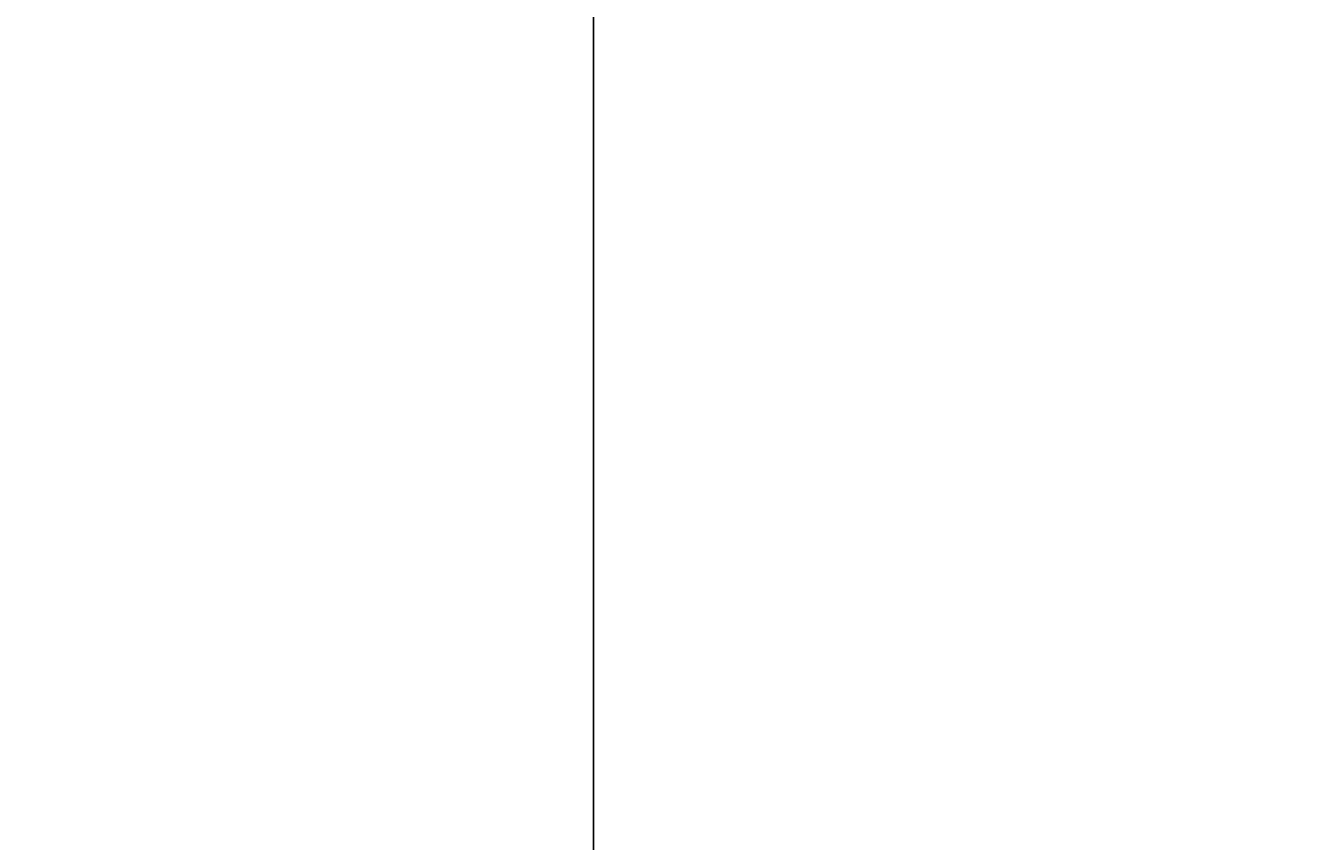
# Model space of a CAD drawing. Units: inches. Extents: x 35362 to 73946, y 43607 to 67532.
# Tile 114 of 134: x 51013 to 51049, y 49015 to 49038. Entities that reach past the tile are written whole.
import ezdxf

# ---------------------------------------------------------------- set-up
doc = ezdxf.new("R2010")
doc.units = ezdxf.units.IN
doc.header["$MEASUREMENT"] = 0
doc.layers.add('A-ANNO-DIMS', color=2, linetype='Continuous', lineweight=18)
doc.styles.get("Standard").update_dxf_attribs({"font": 'arial.ttf'})
doc.dimstyles.get("Standard").update_dxf_attribs({"dimtxt": 0.18, "dimasz": 0.18, "dimexe": 0.18, "dimexo": 0.0625, "dimgap": 0.09, "dimtad": 0, "dimtih": 1, "dimtoh": 1, "dimdec": 4, "dimzin": 0, "dimdsep": 46, "dimtxsty": 'Standard', "dimcen": 0.09, "dimadec": 0, "dimazin": 0, "dimtfac": 1, "dimtdec": 4, "dimtofl": 0, "dimtmove": 0, "dimatfit": 3, "dimfxl": 1, "dimtolj": 1, "dimtzin": 0, "dimarcsym": 0})

# ---------------------------------------------------------------- blocks, each defined once
blk = doc.blocks.new('*D11')
at = {"layer": 'A-ANNO-DIMS', "color": 0, "lineweight": -2, "transparency": 16777216}
for p, q in [((47978.665, 56028.774), (47978.665, 43606.679)), ((53109.76, 56028.774), (53109.76, 43606.679)), ((47978.845, 43606.859), (50543.871, 43606.859)), ((53109.58, 43606.859), (50544.554, 43606.859))]:
    blk.add_line(p, q, dxfattribs=at)
at = {"layer": 'A-ANNO-DIMS', "color": 0, "transparency": 16777216}
for points in [[(47978.845, 43606.889), (47978.845, 43606.829), (47978.665, 43606.859)], [(53109.58, 43606.889), (53109.58, 43606.829), (53109.76, 43606.859)]]:
    blk.add_solid(points, dxfattribs=at)
at = {"layer": 'Defpoints', "color": 0, "transparency": 16777216}
for p in [(47978.665, 56028.836), (53109.76, 56028.836), (53109.76, 43606.859)]:
    blk.add_point(p, dxfattribs=at)
at = {"layer": 'A-ANNO-DIMS', "color": 0, "transparency": 16777216, "insert": (50544.212, 43606.859), "char_height": 0.18, "attachment_point": 5}
blk.add_mtext('\\A1;5131', dxfattribs=at)
blk = doc.blocks.new('*D13')
at = {"layer": 'A-ANNO-DIMS', "color": 0, "lineweight": -2, "transparency": 16777216}
for p, q in [((48373.492, 51694.025), (48373.492, 43606.679)), ((51029.043, 51694.025), (51029.043, 43606.679)), ((48373.672, 43606.859), (49700.802, 43606.859)), ((51028.863, 43606.859), (49701.733, 43606.859))]:
    blk.add_line(p, q, dxfattribs=at)
at = {"layer": 'A-ANNO-DIMS', "color": 0, "transparency": 16777216}
for points in [[(48373.672, 43606.889), (48373.672, 43606.829), (48373.492, 43606.859)], [(51028.863, 43606.889), (51028.863, 43606.829), (51029.043, 43606.859)]]:
    blk.add_solid(points, dxfattribs=at)
at = {"layer": 'Defpoints', "color": 0, "transparency": 16777216}
for p in [(48373.492, 51694.087), (51029.043, 51694.087), (51029.043, 43606.859)]:
    blk.add_point(p, dxfattribs=at)
at = {"layer": 'A-ANNO-DIMS', "color": 0, "transparency": 16777216, "insert": (49701.267, 43606.859), "char_height": 0.18, "attachment_point": 5}
blk.add_mtext('\\A1;2655.6', dxfattribs=at)
blk = doc.blocks.new('*D17')
at = {"layer": 'A-ANNO-DIMS', "color": 0, "lineweight": -2, "transparency": 16777216}
for p, q in [((49923.307, 61293.224), (49923.307, 43606.679)), ((51913.931, 61293.224), (51913.931, 43606.679)), ((49923.487, 43606.859), (50918.164, 43606.859)), ((51913.751, 43606.859), (50919.074, 43606.859))]:
    blk.add_line(p, q, dxfattribs=at)
at = {"layer": 'A-ANNO-DIMS', "color": 0, "transparency": 16777216}
for points in [[(49923.487, 43606.889), (49923.487, 43606.829), (49923.307, 43606.859)], [(51913.751, 43606.889), (51913.751, 43606.829), (51913.931, 43606.859)]]:
    blk.add_solid(points, dxfattribs=at)
at = {"layer": 'Defpoints', "color": 0, "transparency": 16777216}
for p in [(49923.307, 61293.286), (51913.931, 61293.286), (51913.931, 43606.859)]:
    blk.add_point(p, dxfattribs=at)
at = {"layer": 'A-ANNO-DIMS', "color": 0, "transparency": 16777216, "insert": (50918.619, 43606.859), "char_height": 0.18, "attachment_point": 5}
blk.add_mtext('\\A1;1990.6', dxfattribs=at)
blk = doc.blocks.new('*D67')
at = {"layer": 'A-ANNO-DIMS', "color": 0, "lineweight": -2, "transparency": 16777216}
for p, q in [((56873.539, 53351.529), (35361.769, 53351.529)), ((35361.949, 53351.349), (35361.949, 49400.893)), ((35361.949, 45450.074), (35361.949, 49400.53)), ((53793.575, 45449.894), (35361.769, 45449.894))]:
    blk.add_line(p, q, dxfattribs=at)
at = {"layer": 'A-ANNO-DIMS', "color": 0, "transparency": 16777216}
for points in [[(35361.919, 53351.349), (35361.979, 53351.349), (35361.949, 53351.529)], [(35361.919, 45450.074), (35361.979, 45450.074), (35361.949, 45449.894)]]:
    blk.add_solid(points, dxfattribs=at)
at = {"layer": 'Defpoints', "color": 0, "transparency": 16777216}
for p in [(35361.949, 53351.529), (56873.602, 53351.529), (53793.638, 45449.894)]:
    blk.add_point(p, dxfattribs=at)
at = {"layer": 'A-ANNO-DIMS', "color": 0, "transparency": 16777216, "insert": (35361.949, 49400.712), "char_height": 0.18, "attachment_point": 5}
blk.add_mtext('\\A1;7901.6', dxfattribs=at)
blk = doc.blocks.new('*D84')
at = {"layer": 'A-ANNO-DIMS', "color": 0, "lineweight": -2, "transparency": 16777216}
for p, q in [((55540.235, 49259.935), (35361.769, 49259.935)), ((35361.949, 49259.755), (35361.949, 49115.139)), ((35361.949, 48970.16), (35361.949, 49114.776)), ((55540.235, 48969.98), (35361.769, 48969.98))]:
    blk.add_line(p, q, dxfattribs=at)
at = {"layer": 'A-ANNO-DIMS', "color": 0, "transparency": 16777216}
for points in [[(35361.919, 49259.755), (35361.979, 49259.755), (35361.949, 49259.935)], [(35361.919, 48970.16), (35361.979, 48970.16), (35361.949, 48969.98)]]:
    blk.add_solid(points, dxfattribs=at)
at = {"layer": 'Defpoints', "color": 0, "transparency": 16777216}
for p in [(35361.949, 49259.935), (55540.297, 49259.935), (55540.297, 48969.98)]:
    blk.add_point(p, dxfattribs=at)
at = {"layer": 'A-ANNO-DIMS', "color": 0, "transparency": 16777216, "insert": (35361.949, 49114.957), "char_height": 0.18, "attachment_point": 5}
blk.add_mtext('\\A1;289.96', dxfattribs=at)
blk = doc.blocks.new('*D86')
at = {"layer": 'A-ANNO-DIMS', "color": 0, "lineweight": -2, "transparency": 16777216}
for p, q in [((51285.532, 49320.079), (35361.769, 49320.079)), ((35361.949, 49319.899), (35361.949, 49120.261)), ((35361.949, 48920.259), (35361.949, 49119.897)), ((51285.532, 48920.079), (35361.769, 48920.079))]:
    blk.add_line(p, q, dxfattribs=at)
at = {"layer": 'A-ANNO-DIMS', "color": 0, "transparency": 16777216}
for points in [[(35361.919, 49319.899), (35361.979, 49319.899), (35361.949, 49320.079)], [(35361.919, 48920.259), (35361.979, 48920.259), (35361.949, 48920.079)]]:
    blk.add_solid(points, dxfattribs=at)
at = {"layer": 'Defpoints', "color": 0, "transparency": 16777216}
for p in [(35361.949, 49320.079), (51285.595, 49320.079), (51285.595, 48920.079)]:
    blk.add_point(p, dxfattribs=at)
at = {"layer": 'A-ANNO-DIMS', "color": 0, "transparency": 16777216, "insert": (35361.949, 49120.079), "char_height": 0.18, "attachment_point": 5}
blk.add_mtext('\\A1;400.0', dxfattribs=at)
blk = doc.blocks.new('*D107')
at = {"layer": 'A-ANNO-DIMS', "color": 0, "lineweight": -2, "transparency": 16777216}
for p, q in [((50139.563, 59850.014), (50139.563, 43606.679)), ((51320.813, 59850.014), (51320.813, 43606.679)), ((50139.743, 43606.859), (50729.733, 43606.859)), ((51320.633, 43606.859), (50730.643, 43606.859))]:
    blk.add_line(p, q, dxfattribs=at)
at = {"layer": 'A-ANNO-DIMS', "color": 0, "transparency": 16777216}
for points in [[(50139.743, 43606.889), (50139.743, 43606.829), (50139.563, 43606.859)], [(51320.633, 43606.889), (51320.633, 43606.829), (51320.813, 43606.859)]]:
    blk.add_solid(points, dxfattribs=at)
at = {"layer": 'Defpoints', "color": 0, "transparency": 16777216}
for p in [(50139.563, 59850.077), (51320.813, 59850.077), (51320.813, 43606.859)]:
    blk.add_point(p, dxfattribs=at)
at = {"layer": 'A-ANNO-DIMS', "color": 0, "transparency": 16777216, "insert": (50730.188, 43606.859), "char_height": 0.18, "attachment_point": 5}
blk.add_mtext('\\A1;1181.3', dxfattribs=at)

msp = doc.modelspace()

# ---------------------------------------------------------------- dimensions: what is measured, and where the dimension line sits
at = {"layer": 'A-ANNO-DIMS'}
for base, p1, p2, override, picture, middle in [((51913.931, 43606.859), (49923.307, 61293.286), (51913.931, 61293.286), {"dimdec": 1, "dimlfac": 1, "dimrnd": 0, "dimzin": 0, "dimdsep": 46, "dimlunit": 2}, '*D17', (50918.619, 43606.859)), ((51320.8133, 43606.859), (50139.5627, 59850.0769), (51320.8133, 59850.0769), {"dimdec": 1, "dimlfac": 1, "dimrnd": 0, "dimzin": 0, "dimdsep": 46, "dimlunit": 2}, '*D107', (50730.188, 43606.859)), ((53109.76, 43606.859), (47978.665, 56028.836), (53109.76, 56028.836), {"dimdec": 0, "dimlfac": 1, "dimrnd": 0, "dimzin": 0, "dimdsep": 46, "dimlunit": 2}, '*D11', (50544.212, 43606.859)), ((51029.043, 43606.859), (48373.492, 51694.087), (51029.043, 51694.087), {"dimdec": 1, "dimlfac": 1, "dimrnd": 0, "dimzin": 0, "dimdsep": 46, "dimlunit": 2}, '*D13', (49701.267, 43606.859))]:
    dim = msp.add_linear_dim(base=base, p1=p1, p2=p2, dimstyle='Standard', override=override, dxfattribs=at)
    dim.commit()
    dim.dimension.update_dxf_attribs({"geometry": picture, "text_midpoint": middle})
for base, p1, p2, override, picture, middle in [((35361.949, 53351.529), (53793.638, 45449.894), (56873.602, 53351.529), {"dimdec": 1, "dimlfac": 1, "dimrnd": 0, "dimzin": 0, "dimdsep": 46, "dimlunit": 2}, '*D67', (35361.949, 49400.712)), ((35361.949, 49320.079), (51285.595, 48920.079), (51285.595, 49320.079), {"dimdec": 1, "dimlfac": 1, "dimrnd": 0, "dimzin": 0, "dimdsep": 46, "dimlunit": 2}, '*D86', (35361.949, 49120.079)), ((35361.9491, 49259.9353), (55540.2972, 48969.9796), (55540.2972, 49259.9353), {"dimdec": 2, "dimlfac": 1, "dimrnd": 0, "dimzin": 0, "dimdsep": 46, "dimlunit": 2}, '*D84', (35361.9491, 49114.9575))]:
    dim = msp.add_linear_dim(base=base, p1=p1, p2=p2, angle=90, dimstyle='Standard', override=override, dxfattribs=at)
    dim.commit()
    dim.dimension.update_dxf_attribs({"geometry": picture, "text_midpoint": middle})

doc.saveas('drawing.dxf')
